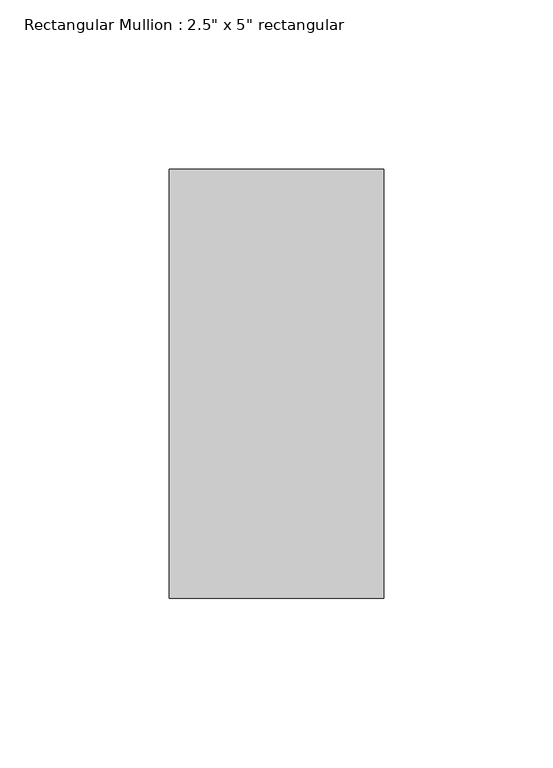
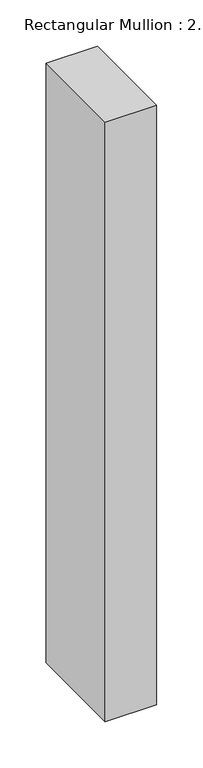
"""IFC4 building model written with IfcOpenShell, lengths in millimetres: member geometry."""

from ifc_helpers import new_model, si_unit, frame, origin, place, context, project, spatial, polyline, outline, extrude, source, transform, mapped, element, save


def member_429f6687(model_context):
    return source(origin(), model_context, "Body", "SweptSolid", [
        extrude(outline(polyline([(0.0, 63.5), (0.0, -63.5), (-63.5, -63.5), (-63.5, 63.5), (0.0, 63.5)])), frame((0.0, 0.0, -787.4), z_axis=(0.0, 0.0, 1.0), x_axis=(1.0, 0.0, 0.0)), (0.0, 0.0, 1.0), 787.4),
    ])


if __name__ == "__main__":
    model = new_model("IFC4")
    model_context = context("Model", 3, world=origin())
    ifc_project = project(units=[si_unit("LENGTHUNIT", "METRE", prefix="MILLI")], contexts=[model_context])
    site = spatial("IfcSite", under=ifc_project)
    building = spatial("IfcBuilding", under=site)
    placement = place(None, origin())
    member_shape = member_429f6687(model_context)
    element("IfcMember", 1, ObjectType="Rectangular Mullion : 2.5\" x 5\" rectangular", at=placement, inside=building, context=model_context, shape_type="MappedRepresentation", body=[
        mapped(member_shape, transform((0.0, 0.0, 0.0), x_axis=(1.0, 0.0, 0.0), y_axis=(0.0, 1.0, 0.0), z_axis=(0.0, 0.0, 1.0))),
    ])
    save(model, "model.ifc")

# Revit data of these elements
# Type "Rectangular Mullion : 2.5\" x 5\" rectangular"
#   built-in parameter 1007304 = 0.416667 (stored number, unit not read)
#   built-in parameter 1007301 = 0.104167 (stored number, unit not read)
#   built-in parameter 1007300 = 0.104167 (stored number, unit not read)
# Element 1 (IfcMember, "Rectangular Mullion : 2.5\" x 5\" rectangular")
#   Materials on its faces: "Aluminum"
# Materials
#   "Aluminum": class "Metal", colour RGB 247 247 247, transparency 0, Description = "Aluminum 6061", Cost = 0
